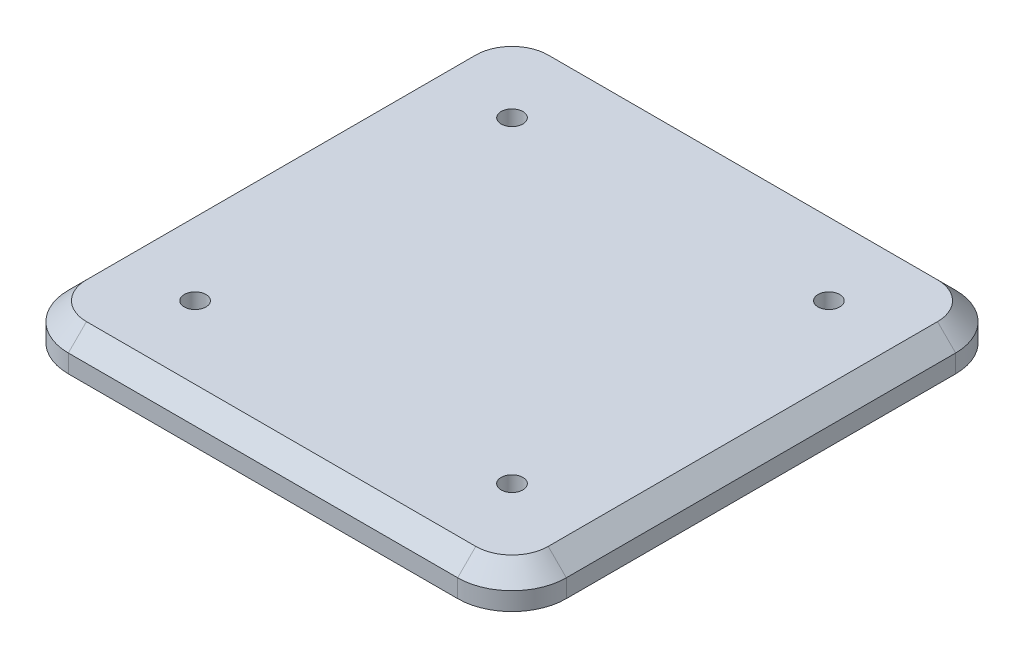
SolidWorks part; units mm, degrees
material "Plain Carbon Steel"
ref_plane "Front Plane" through (0, 0, 0) normal (0, 0, 1) x (1, 0, 0)
ref_plane "Top Plane" through (0, 0, 0) normal (0, 1, 0) x (1, 0, 0)
ref_plane "Right Plane" through (0, 0, 0) normal (1, 0, 0) x (0, 0, -1)
sketch "Base Plate Profile 275x275" plane through (0, 0, 0) normal (0, 1, 0) x (1, 0, 0)
  line L1 (-137.5, -137.5) -> (137.5, -137.5)
  line L2 (-137.5, -137.5) -> (-137.5, 137.5)
  line L3 (-137.5, 137.5) -> (137.5, 137.5)
  line L4 (137.5, -137.5) -> (137.5, 137.5)
  line L5 (-137.5, -137.5) -> (137.5, 137.5) construction
  line L6 (-137.5, 137.5) -> (137.5, -137.5) construction
  point P0 (0, 0)
  dimension "D1" = 275
  dimension "D2" = 275
extrude "Base Plate 275x275x20" add sketch "Base Plate Profile 275x275" along normal blind 20 contours L2 L3 L4 L1
fillet "Corner Fillets R30" radius 30 4 edges at (137.5, 10, -137.5) (-137.5, 10, -137.5) (137.5, 10, 137.5) (-137.5, 10, 137.5)
chamfer "Edge Chamfer 10x45" distance 10 angle 45 8 edges at (0, 20, -137.5) (-128.7132, 20, -128.7132) (128.7132, 20, -128.7132) (-137.5, 20, 0) (137.5, 20, 0) (-128.7132, 20, 128.7132) (128.7132, 20, 128.7132) (0, 20, 137.5)
sketch "Dowel Hole Layout 175 Square" plane through (0, 20, 0) normal (0, 1, 0) x (1, 0, 0)
  line L1 (-87.5, -87.5) -> (87.5, -87.5)
  line L2 (-87.5, -87.5) -> (-87.5, 87.5)
  line L3 (-87.5, 87.5) -> (87.5, 87.5)
  line L4 (87.5, -87.5) -> (87.5, 87.5)
  line L5 (-87.5, -87.5) -> (87.5, 87.5) construction
  line L6 (-87.5, 87.5) -> (87.5, -87.5) construction
  point P0 (0, 0)
  dimension "D1" = 175
  dimension "D2" = 175
hole_wizard "Dowel Holes Ø12 on 175 Square" positions "3DSketch1" profile "Sketch3" hole size "Ø12.0" standard "ANSI Metric"
sketch3d "3DSketch1"
  point P0 (-87.5, 20, -87.5)
  point P3 (87.5, 20, -87.5)
  point P6 (87.5, 20, 87.5)
  point P9 (-87.5, 20, 87.5)
sketch "Sketch3" plane through (-87.5, 20, -87.5) normal (1, 0, 0) x (0, 0, 1)
  line L0 (0, 0) -> (0, 13.6052)
  line L1 (0, 13.6052) -> (6, 10)
  line L2 (6, 10) -> (6, 0)
  line L5 (6, 0) -> (0, 0)
  line L10 (0, 13.6052) -> (-6, 10) construction
  line L11 (0, -6.35) -> (0, 107.95) construction
  dimension "Hole Dia." = 12
  dimension "Hole Depth" = 10
  dimension "Drill Angle" = 118
sketch "Dowel Hole Layout 225 Square" plane through (0, 0, 0) normal (0, -1, 0) x (1, 0, 0)
  line L1 (-112.5, -112.5) -> (112.5, -112.5)
  line L2 (-112.5, -112.5) -> (-112.5, 112.5)
  line L3 (-112.5, 112.5) -> (112.5, 112.5)
  line L4 (112.5, -112.5) -> (112.5, 112.5)
  line L5 (-112.5, -112.5) -> (112.5, 112.5) construction
  line L6 (-112.5, 112.5) -> (112.5, -112.5) construction
  point P0 (0, 0)
  dimension "D1" = 225
  dimension "D2" = 225
hole_wizard "Dowel Holes Ø12 on 225 Square" positions "3DSketch2" profile "Sketch5" hole size "Ø12.0" standard "ANSI Metric"
sketch3d "3DSketch2"
  point P0 (-112.5, 0, 112.5)
  point P3 (112.5, 0, 112.5)
  point P6 (112.5, 0, -112.5)
  point P9 (-112.5, 0, -112.5)
sketch "Sketch5" plane through (-112.5, 0, 112.5) normal (1, 0, 0) x (0, 0, -1)
  line L0 (0, 0) -> (0, 13.6052)
  line L1 (0, 13.6052) -> (6, 10)
  line L2 (6, 10) -> (6, 0)
  line L5 (6, 0) -> (0, 0)
  line L10 (0, 13.6052) -> (-6, 10) construction
  line L11 (0, -6.35) -> (0, 107.95) construction
  dimension "Hole Dia." = 12
  dimension "Hole Depth" = 10
  dimension "Drill Angle" = 118
